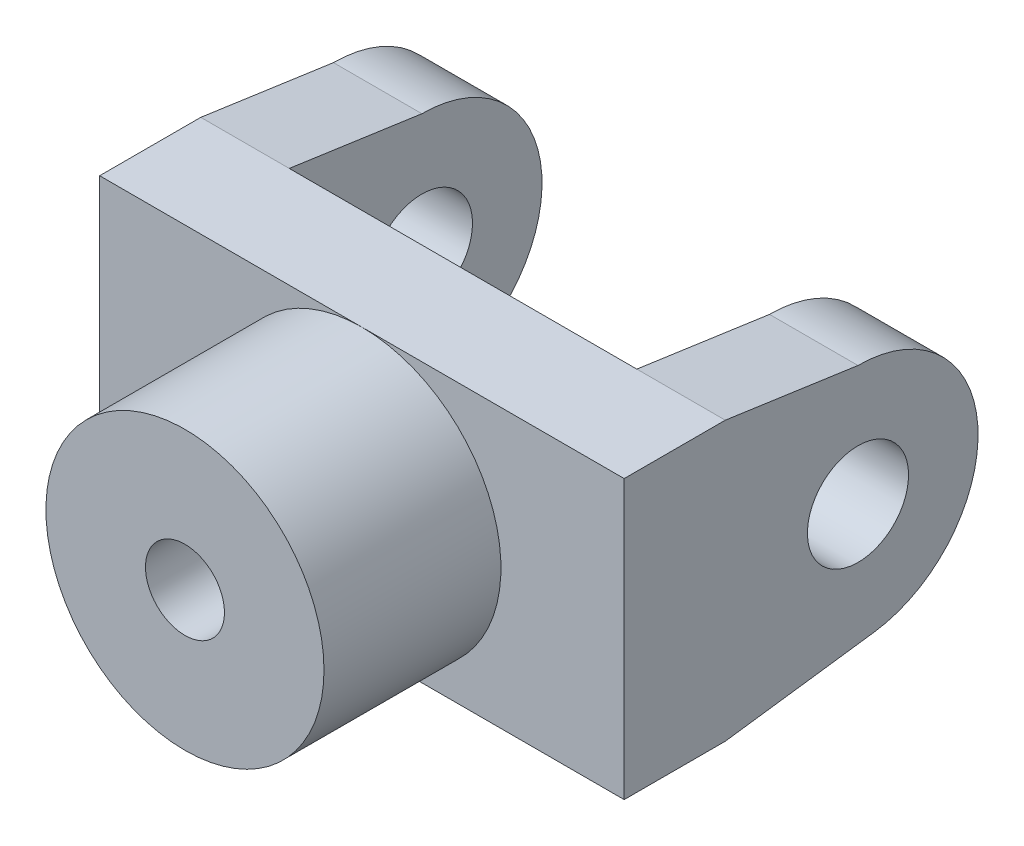
ISO-10303-21;
HEADER;
FILE_DESCRIPTION(('STEP AP214'),'2;1');
FILE_NAME('part.step','',(''),(''),'','','');
FILE_SCHEMA(('AUTOMOTIVE_DESIGN { 1 0 10303 214 1 1 1 1 }'));
ENDSEC;
DATA;
#1=APPLICATION_CONTEXT('core data for automotive mechanical design processes');
#2=APPLICATION_PROTOCOL_DEFINITION('international standard','automotive_design',2000,#1);
#3=PRODUCT_CONTEXT('',#1,'mechanical');
#4=PRODUCT('Part','Part','',(#3));
#5=PRODUCT_RELATED_PRODUCT_CATEGORY('part','',(#4));
#6=PRODUCT_DEFINITION_FORMATION('','',#4);
#7=PRODUCT_DEFINITION_CONTEXT('part definition',#1,'design');
#8=PRODUCT_DEFINITION('design','',#6,#7);
#9=PRODUCT_DEFINITION_SHAPE('','',#8);
#10=(LENGTH_UNIT() NAMED_UNIT(*) SI_UNIT(.MILLI.,.METRE.));
#11=(NAMED_UNIT(*) PLANE_ANGLE_UNIT() SI_UNIT($,.RADIAN.));
#12=(NAMED_UNIT(*) SI_UNIT($,.STERADIAN.) SOLID_ANGLE_UNIT());
#13=UNCERTAINTY_MEASURE_WITH_UNIT(LENGTH_MEASURE(1.E-05),#10,'distance_accuracy_value','');
#14=(GEOMETRIC_REPRESENTATION_CONTEXT(3) GLOBAL_UNCERTAINTY_ASSIGNED_CONTEXT((#13)) GLOBAL_UNIT_ASSIGNED_CONTEXT((#10,
#11,#12)) REPRESENTATION_CONTEXT('',''));
#15=CARTESIAN_POINT('',(0.,0.,0.));
#16=DIRECTION('',(0.,0.,1.));
#17=DIRECTION('',(1.,0.,0.));
#18=AXIS2_PLACEMENT_3D('',#15,#16,#17);
#19=CARTESIAN_POINT('',(0.,0.,0.));
#20=DIRECTION('',(0.,0.,1.));
#21=DIRECTION('',(1.,0.,0.));
#22=AXIS2_PLACEMENT_3D('',#19,#20,#21);
#23=PLANE('',#22);
#24=DIRECTION('',(0.,-1.,0.));
#25=VECTOR('',#24,1.);
#26=CARTESIAN_POINT('',(-55.,44.,0.));
#27=LINE('',#26,#25);
#28=CARTESIAN_POINT('',(-55.,44.,0.));
#29=VERTEX_POINT('',#28);
#30=CARTESIAN_POINT('',(-55.,-44.,0.));
#31=VERTEX_POINT('',#30);
#32=EDGE_CURVE('E141',#29,#31,#27,.T.);
#33=ORIENTED_EDGE('',*,*,#32,.F.);
#34=DIRECTION('',(-1.,0.,0.));
#35=VECTOR('',#34,1.);
#36=CARTESIAN_POINT('',(83.,44.,0.));
#37=LINE('',#36,#35);
#38=CARTESIAN_POINT('',(55.,44.,0.));
#39=VERTEX_POINT('',#38);
#40=EDGE_CURVE('E224',#39,#29,#37,.T.);
#41=ORIENTED_EDGE('',*,*,#40,.F.);
#42=DIRECTION('',(0.,-1.,0.));
#43=VECTOR('',#42,1.);
#44=CARTESIAN_POINT('',(55.,44.,0.));
#45=LINE('',#44,#43);
#46=CARTESIAN_POINT('',(55.,-44.,0.));
#47=VERTEX_POINT('',#46);
#48=EDGE_CURVE('E172',#39,#47,#45,.T.);
#49=ORIENTED_EDGE('',*,*,#48,.T.);
#50=DIRECTION('',(1.,0.,0.));
#51=VECTOR('',#50,1.);
#52=CARTESIAN_POINT('',(83.,-44.,0.));
#53=LINE('',#52,#51);
#54=EDGE_CURVE('E62',#31,#47,#53,.T.);
#55=ORIENTED_EDGE('',*,*,#54,.F.);
#56=EDGE_LOOP('',(#33,#41,#49,#55));
#57=FACE_BOUND('',#56,.T.);
#58=ADVANCED_FACE('F39',(#57),#23,.F.);
#59=CARTESIAN_POINT('',(0.,0.,32.));
#60=DIRECTION('',(0.,0.,1.));
#61=DIRECTION('',(1.,0.,0.));
#62=AXIS2_PLACEMENT_3D('',#59,#60,#61);
#63=PLANE('',#62);
#64=CARTESIAN_POINT('',(0.,0.,32.));
#65=DIRECTION('',(0.,0.,1.));
#66=DIRECTION('',(1.,0.,0.));
#67=AXIS2_PLACEMENT_3D('',#64,#65,#66);
#68=CIRCLE('',#67,44.);
#69=CARTESIAN_POINT('',(0.,44.,32.));
#70=VERTEX_POINT('',#69);
#71=CARTESIAN_POINT('',(0.,-44.,32.));
#72=VERTEX_POINT('',#71);
#73=EDGE_CURVE('E47',#70,#72,#68,.T.);
#74=ORIENTED_EDGE('',*,*,#73,.F.);
#75=DIRECTION('',(-1.,0.,0.));
#76=VECTOR('',#75,1.);
#77=CARTESIAN_POINT('',(83.,44.,32.));
#78=LINE('',#77,#76);
#79=CARTESIAN_POINT('',(-83.,44.,32.));
#80=VERTEX_POINT('',#79);
#81=EDGE_CURVE('E220',#70,#80,#78,.T.);
#82=ORIENTED_EDGE('',*,*,#81,.T.);
#83=DIRECTION('',(0.,-1.,0.));
#84=VECTOR('',#83,1.);
#85=CARTESIAN_POINT('',(-83.,-44.,32.));
#86=LINE('',#85,#84);
#87=CARTESIAN_POINT('',(-83.,-44.,32.));
#88=VERTEX_POINT('',#87);
#89=EDGE_CURVE('E210',#80,#88,#86,.T.);
#90=ORIENTED_EDGE('',*,*,#89,.T.);
#91=DIRECTION('',(1.,0.,0.));
#92=VECTOR('',#91,1.);
#93=CARTESIAN_POINT('',(83.,-44.,32.));
#94=LINE('',#93,#92);
#95=EDGE_CURVE('E215',#88,#72,#94,.T.);
#96=ORIENTED_EDGE('',*,*,#95,.T.);
#97=EDGE_LOOP('',(#74,#82,#90,#96));
#98=FACE_BOUND('',#97,.T.);
#99=ADVANCED_FACE('F254',(#98),#63,.T.);
#100=CARTESIAN_POINT('',(-83.,-44.,32.));
#101=DIRECTION('',(1.,0.,0.));
#102=DIRECTION('',(0.,0.,-1.));
#103=AXIS2_PLACEMENT_3D('',#100,#101,#102);
#104=PLANE('',#103);
#105=DIRECTION('',(0.,0.,-1.));
#106=VECTOR('',#105,1.);
#107=CARTESIAN_POINT('',(-83.,44.,32.));
#108=LINE('',#107,#106);
#109=CARTESIAN_POINT('',(-83.,44.,0.));
#110=VERTEX_POINT('',#109);
#111=EDGE_CURVE('E219',#80,#110,#108,.T.);
#112=ORIENTED_EDGE('',*,*,#111,.T.);
#113=DIRECTION('',(0.,0.141421356237309,0.989949493661166));
#114=VECTOR('',#113,1.);
#115=CARTESIAN_POINT('',(-83.,38.,-42.));
#116=LINE('',#115,#114);
#117=CARTESIAN_POINT('',(-83.,38.,-42.));
#118=VERTEX_POINT('',#117);
#119=EDGE_CURVE('E158',#118,#110,#116,.T.);
#120=ORIENTED_EDGE('',*,*,#119,.F.);
#121=CARTESIAN_POINT('',(-83.,0.,-42.));
#122=DIRECTION('',(1.,0.,0.));
#123=DIRECTION('',(0.,0.,-1.));
#124=AXIS2_PLACEMENT_3D('',#121,#122,#123);
#125=CIRCLE('',#124,38.);
#126=CARTESIAN_POINT('',(-83.,-37.6599459145,-47.072324291381));
#127=VERTEX_POINT('',#126);
#128=EDGE_CURVE('E137',#127,#118,#125,.T.);
#129=ORIENTED_EDGE('',*,*,#128,.F.);
#130=DIRECTION('',(0.,0.133482218194236,-0.991051208276316));
#131=VECTOR('',#130,1.);
#132=CARTESIAN_POINT('',(-83.,-44.,0.));
#133=LINE('',#132,#131);
#134=CARTESIAN_POINT('',(-83.,-44.,0.));
#135=VERTEX_POINT('',#134);
#136=EDGE_CURVE('E149',#135,#127,#133,.T.);
#137=ORIENTED_EDGE('',*,*,#136,.F.);
#138=DIRECTION('',(0.,0.,-1.));
#139=VECTOR('',#138,1.);
#140=CARTESIAN_POINT('',(-83.,-44.,32.));
#141=LINE('',#140,#139);
#142=EDGE_CURVE('E43',#88,#135,#141,.T.);
#143=ORIENTED_EDGE('',*,*,#142,.F.);
#144=ORIENTED_EDGE('',*,*,#89,.F.);
#145=EDGE_LOOP('',(#112,#120,#129,#137,#143,#144));
#146=FACE_BOUND('',#145,.T.);
#147=CARTESIAN_POINT('',(-83.,0.,-42.));
#148=DIRECTION('',(1.,0.,0.));
#149=DIRECTION('',(0.,0.,-1.));
#150=AXIS2_PLACEMENT_3D('',#147,#148,#149);
#151=CIRCLE('',#150,16.);
#152=CARTESIAN_POINT('',(-83.,0.,-58.));
#153=VERTEX_POINT('',#152);
#154=EDGE_CURVE('E153',#153,#153,#151,.T.);
#155=ORIENTED_EDGE('',*,*,#154,.T.);
#156=EDGE_LOOP('',(#155));
#157=FACE_BOUND('',#156,.T.);
#158=ADVANCED_FACE('F41',(#146,#157),#104,.F.);
#159=CARTESIAN_POINT('',(83.,-44.,32.));
#160=DIRECTION('',(0.,1.,0.));
#161=DIRECTION('',(-1.,0.,0.));
#162=AXIS2_PLACEMENT_3D('',#159,#160,#161);
#163=PLANE('',#162);
#164=EDGE_CURVE('E222',#135,#31,#53,.T.);
#165=ORIENTED_EDGE('',*,*,#164,.T.);
#166=ORIENTED_EDGE('',*,*,#54,.T.);
#167=DIRECTION('',(1.,0.,0.));
#168=VECTOR('',#167,1.);
#169=CARTESIAN_POINT('',(55.,-44.,0.));
#170=LINE('',#169,#168);
#171=CARTESIAN_POINT('',(83.,-44.,0.));
#172=VERTEX_POINT('',#171);
#173=EDGE_CURVE('E184',#47,#172,#170,.T.);
#174=ORIENTED_EDGE('',*,*,#173,.T.);
#175=DIRECTION('',(0.,0.,-1.));
#176=VECTOR('',#175,1.);
#177=CARTESIAN_POINT('',(83.,-44.,32.));
#178=LINE('',#177,#176);
#179=CARTESIAN_POINT('',(83.,-44.,32.));
#180=VERTEX_POINT('',#179);
#181=EDGE_CURVE('E229',#180,#172,#178,.T.);
#182=ORIENTED_EDGE('',*,*,#181,.F.);
#183=EDGE_CURVE('E209',#72,#180,#94,.T.);
#184=ORIENTED_EDGE('',*,*,#183,.F.);
#185=ORIENTED_EDGE('',*,*,#95,.F.);
#186=ORIENTED_EDGE('',*,*,#142,.T.);
#187=EDGE_LOOP('',(#165,#166,#174,#182,#184,#185,#186));
#188=FACE_BOUND('',#187,.T.);
#189=ADVANCED_FACE('F240',(#188),#163,.F.);
#190=CARTESIAN_POINT('',(83.,-44.,32.));
#191=DIRECTION('',(-1.,0.,0.));
#192=DIRECTION('',(0.,0.,1.));
#193=AXIS2_PLACEMENT_3D('',#190,#191,#192);
#194=PLANE('',#193);
#195=ORIENTED_EDGE('',*,*,#181,.T.);
#196=DIRECTION('',(0.,0.133482218194236,-0.991051208276316));
#197=VECTOR('',#196,1.);
#198=CARTESIAN_POINT('',(83.,-44.,0.));
#199=LINE('',#198,#197);
#200=CARTESIAN_POINT('',(83.,-37.6599459145,-47.072324291381));
#201=VERTEX_POINT('',#200);
#202=EDGE_CURVE('E190',#172,#201,#199,.T.);
#203=ORIENTED_EDGE('',*,*,#202,.T.);
#204=CARTESIAN_POINT('',(83.,0.,-42.));
#205=DIRECTION('',(1.,0.,0.));
#206=DIRECTION('',(0.,0.,-1.));
#207=AXIS2_PLACEMENT_3D('',#204,#205,#206);
#208=CIRCLE('',#207,38.);
#209=CARTESIAN_POINT('',(83.,38.,-42.));
#210=VERTEX_POINT('',#209);
#211=EDGE_CURVE('E174',#201,#210,#208,.T.);
#212=ORIENTED_EDGE('',*,*,#211,.T.);
#213=DIRECTION('',(0.,0.141421356237309,0.989949493661166));
#214=VECTOR('',#213,1.);
#215=CARTESIAN_POINT('',(83.,38.,-42.));
#216=LINE('',#215,#214);
#217=CARTESIAN_POINT('',(83.,44.,0.));
#218=VERTEX_POINT('',#217);
#219=EDGE_CURVE('E169',#210,#218,#216,.T.);
#220=ORIENTED_EDGE('',*,*,#219,.T.);
#221=DIRECTION('',(0.,0.,-1.));
#222=VECTOR('',#221,1.);
#223=CARTESIAN_POINT('',(83.,44.,32.));
#224=LINE('',#223,#222);
#225=CARTESIAN_POINT('',(83.,44.,32.));
#226=VERTEX_POINT('',#225);
#227=EDGE_CURVE('E226',#226,#218,#224,.T.);
#228=ORIENTED_EDGE('',*,*,#227,.F.);
#229=DIRECTION('',(0.,1.,0.));
#230=VECTOR('',#229,1.);
#231=CARTESIAN_POINT('',(83.,-44.,32.));
#232=LINE('',#231,#230);
#233=EDGE_CURVE('E214',#180,#226,#232,.T.);
#234=ORIENTED_EDGE('',*,*,#233,.F.);
#235=EDGE_LOOP('',(#195,#203,#212,#220,#228,#234));
#236=FACE_BOUND('',#235,.T.);
#237=CARTESIAN_POINT('',(83.,0.,-42.));
#238=DIRECTION('',(1.,0.,0.));
#239=DIRECTION('',(0.,0.,-1.));
#240=AXIS2_PLACEMENT_3D('',#237,#238,#239);
#241=CIRCLE('',#240,16.);
#242=CARTESIAN_POINT('',(83.,0.,-58.));
#243=VERTEX_POINT('',#242);
#244=EDGE_CURVE('E162',#243,#243,#241,.T.);
#245=ORIENTED_EDGE('',*,*,#244,.F.);
#246=EDGE_LOOP('',(#245));
#247=FACE_BOUND('',#246,.T.);
#248=ADVANCED_FACE('F275',(#236,#247),#194,.F.);
#249=CARTESIAN_POINT('',(83.,44.,32.));
#250=DIRECTION('',(0.,-1.,0.));
#251=DIRECTION('',(1.,0.,0.));
#252=AXIS2_PLACEMENT_3D('',#249,#250,#251);
#253=PLANE('',#252);
#254=EDGE_CURVE('E211',#218,#39,#37,.T.);
#255=ORIENTED_EDGE('',*,*,#254,.T.);
#256=ORIENTED_EDGE('',*,*,#40,.T.);
#257=DIRECTION('',(-1.,0.,0.));
#258=VECTOR('',#257,1.);
#259=CARTESIAN_POINT('',(-55.,44.,0.));
#260=LINE('',#259,#258);
#261=EDGE_CURVE('E150',#29,#110,#260,.T.);
#262=ORIENTED_EDGE('',*,*,#261,.T.);
#263=ORIENTED_EDGE('',*,*,#111,.F.);
#264=ORIENTED_EDGE('',*,*,#81,.F.);
#265=EDGE_CURVE('E217',#226,#70,#78,.T.);
#266=ORIENTED_EDGE('',*,*,#265,.F.);
#267=ORIENTED_EDGE('',*,*,#227,.T.);
#268=EDGE_LOOP('',(#255,#256,#262,#263,#264,#266,#267));
#269=FACE_BOUND('',#268,.T.);
#270=ADVANCED_FACE('F267',(#269),#253,.F.);
#271=EDGE_CURVE('E11',#72,#70,#68,.T.);
#272=ORIENTED_EDGE('',*,*,#271,.F.);
#273=ORIENTED_EDGE('',*,*,#183,.T.);
#274=ORIENTED_EDGE('',*,*,#233,.T.);
#275=ORIENTED_EDGE('',*,*,#265,.T.);
#276=EDGE_LOOP('',(#272,#273,#274,#275));
#277=FACE_BOUND('',#276,.T.);
#278=ADVANCED_FACE('F266',(#277),#63,.T.);
#279=CARTESIAN_POINT('',(0.,0.,88.));
#280=DIRECTION('',(0.,0.,1.));
#281=DIRECTION('',(1.,0.,0.));
#282=AXIS2_PLACEMENT_3D('',#279,#280,#281);
#283=PLANE('',#282);
#284=CARTESIAN_POINT('',(0.,0.,88.));
#285=DIRECTION('',(0.,0.,1.));
#286=DIRECTION('',(1.,0.,0.));
#287=AXIS2_PLACEMENT_3D('',#284,#285,#286);
#288=CIRCLE('',#287,44.);
#289=CARTESIAN_POINT('',(44.,0.,88.));
#290=VERTEX_POINT('',#289);
#291=EDGE_CURVE('E201',#290,#290,#288,.T.);
#292=ORIENTED_EDGE('',*,*,#291,.T.);
#293=EDGE_LOOP('',(#292));
#294=FACE_BOUND('',#293,.T.);
#295=CARTESIAN_POINT('',(0.,0.,88.));
#296=DIRECTION('',(0.,0.,1.));
#297=DIRECTION('',(1.,0.,0.));
#298=AXIS2_PLACEMENT_3D('',#295,#296,#297);
#299=CIRCLE('',#298,12.5);
#300=CARTESIAN_POINT('',(12.5,0.,88.));
#301=VERTEX_POINT('',#300);
#302=EDGE_CURVE('E196',#301,#301,#299,.T.);
#303=ORIENTED_EDGE('',*,*,#302,.F.);
#304=EDGE_LOOP('',(#303));
#305=FACE_BOUND('',#304,.T.);
#306=ADVANCED_FACE('F344',(#294,#305),#283,.T.);
#307=CARTESIAN_POINT('',(0.,0.,88.));
#308=DIRECTION('',(0.,0.,-1.));
#309=DIRECTION('',(-1.,0.,0.));
#310=AXIS2_PLACEMENT_3D('',#307,#308,#309);
#311=CYLINDRICAL_SURFACE('',#310,44.);
#312=ORIENTED_EDGE('',*,*,#291,.F.);
#313=EDGE_LOOP('',(#312));
#314=FACE_BOUND('',#313,.T.);
#315=ORIENTED_EDGE('',*,*,#73,.T.);
#316=ORIENTED_EDGE('',*,*,#271,.T.);
#317=EDGE_LOOP('',(#315,#316));
#318=FACE_BOUND('',#317,.T.);
#319=ADVANCED_FACE('F366',(#314,#318),#311,.T.);
#320=CARTESIAN_POINT('',(0.,0.,88.));
#321=DIRECTION('',(0.,0.,-1.));
#322=DIRECTION('',(-1.,0.,0.));
#323=AXIS2_PLACEMENT_3D('',#320,#321,#322);
#324=CYLINDRICAL_SURFACE('',#323,12.5);
#325=ORIENTED_EDGE('',*,*,#302,.T.);
#326=EDGE_LOOP('',(#325));
#327=FACE_BOUND('',#326,.T.);
#328=CARTESIAN_POINT('',(0.,0.,32.));
#329=DIRECTION('',(0.,0.,1.));
#330=DIRECTION('',(1.,0.,0.));
#331=AXIS2_PLACEMENT_3D('',#328,#329,#330);
#332=CIRCLE('',#331,12.5);
#333=CARTESIAN_POINT('',(12.5,0.,32.));
#334=VERTEX_POINT('',#333);
#335=EDGE_CURVE('E192',#334,#334,#332,.T.);
#336=ORIENTED_EDGE('',*,*,#335,.F.);
#337=EDGE_LOOP('',(#336));
#338=FACE_BOUND('',#337,.T.);
#339=ADVANCED_FACE('F358',(#327,#338),#324,.F.);
#340=ORIENTED_EDGE('',*,*,#335,.T.);
#341=EDGE_LOOP('',(#340));
#342=FACE_BOUND('',#341,.T.);
#343=ADVANCED_FACE('F264',(#342),#63,.T.);
#344=CARTESIAN_POINT('',(55.,38.,-42.));
#345=DIRECTION('',(0.,0.989949493661167,-0.141421356237309));
#346=DIRECTION('',(0.,0.141421356237309,0.989949493661167));
#347=AXIS2_PLACEMENT_3D('',#344,#345,#346);
#348=PLANE('',#347);
#349=ORIENTED_EDGE('',*,*,#219,.F.);
#350=DIRECTION('',(1.,0.,0.));
#351=VECTOR('',#350,1.);
#352=CARTESIAN_POINT('',(55.,38.,-42.));
#353=LINE('',#352,#351);
#354=CARTESIAN_POINT('',(55.,38.,-42.));
#355=VERTEX_POINT('',#354);
#356=EDGE_CURVE('E195',#355,#210,#353,.T.);
#357=ORIENTED_EDGE('',*,*,#356,.F.);
#358=DIRECTION('',(0.,0.141421356237309,0.989949493661166));
#359=VECTOR('',#358,1.);
#360=CARTESIAN_POINT('',(55.,38.,-42.));
#361=LINE('',#360,#359);
#362=EDGE_CURVE('E173',#355,#39,#361,.T.);
#363=ORIENTED_EDGE('',*,*,#362,.T.);
#364=ORIENTED_EDGE('',*,*,#254,.F.);
#365=EDGE_LOOP('',(#349,#357,#363,#364));
#366=FACE_BOUND('',#365,.T.);
#367=ADVANCED_FACE('F354',(#366),#348,.T.);
#368=CARTESIAN_POINT('',(55.,0.,-42.));
#369=DIRECTION('',(1.,0.,0.));
#370=DIRECTION('',(0.,0.,-1.));
#371=AXIS2_PLACEMENT_3D('',#368,#369,#370);
#372=CYLINDRICAL_SURFACE('',#371,38.);
#373=ORIENTED_EDGE('',*,*,#211,.F.);
#374=DIRECTION('',(1.,0.,0.));
#375=VECTOR('',#374,1.);
#376=CARTESIAN_POINT('',(55.,-37.6599459145,-47.072324291381));
#377=LINE('',#376,#375);
#378=CARTESIAN_POINT('',(55.,-37.6599459145,-47.072324291381));
#379=VERTEX_POINT('',#378);
#380=EDGE_CURVE('E194',#379,#201,#377,.T.);
#381=ORIENTED_EDGE('',*,*,#380,.F.);
#382=CARTESIAN_POINT('',(55.,0.,-42.));
#383=DIRECTION('',(1.,0.,0.));
#384=DIRECTION('',(0.,0.,-1.));
#385=AXIS2_PLACEMENT_3D('',#382,#383,#384);
#386=CIRCLE('',#385,38.);
#387=EDGE_CURVE('E182',#379,#355,#386,.T.);
#388=ORIENTED_EDGE('',*,*,#387,.T.);
#389=ORIENTED_EDGE('',*,*,#356,.T.);
#390=EDGE_LOOP('',(#373,#381,#388,#389));
#391=FACE_BOUND('',#390,.T.);
#392=ADVANCED_FACE('F396',(#391),#372,.T.);
#393=CARTESIAN_POINT('',(55.,-44.,0.));
#394=DIRECTION('',(0.,-0.991051208276316,-0.133482218194236));
#395=DIRECTION('',(0.,0.133482218194236,-0.991051208276316));
#396=AXIS2_PLACEMENT_3D('',#393,#394,#395);
#397=PLANE('',#396);
#398=ORIENTED_EDGE('',*,*,#202,.F.);
#399=ORIENTED_EDGE('',*,*,#173,.F.);
#400=DIRECTION('',(0.,0.133482218194236,-0.991051208276316));
#401=VECTOR('',#400,1.);
#402=CARTESIAN_POINT('',(55.,-44.,0.));
#403=LINE('',#402,#401);
#404=EDGE_CURVE('E176',#47,#379,#403,.T.);
#405=ORIENTED_EDGE('',*,*,#404,.T.);
#406=ORIENTED_EDGE('',*,*,#380,.T.);
#407=EDGE_LOOP('',(#398,#399,#405,#406));
#408=FACE_BOUND('',#407,.T.);
#409=ADVANCED_FACE('F406',(#408),#397,.T.);
#410=CARTESIAN_POINT('',(55.,0.,-42.));
#411=DIRECTION('',(1.,0.,0.));
#412=DIRECTION('',(0.,0.,-1.));
#413=AXIS2_PLACEMENT_3D('',#410,#411,#412);
#414=PLANE('',#413);
#415=CARTESIAN_POINT('',(55.,0.,-42.));
#416=DIRECTION('',(1.,0.,0.));
#417=DIRECTION('',(0.,0.,-1.));
#418=AXIS2_PLACEMENT_3D('',#415,#416,#417);
#419=CIRCLE('',#418,16.);
#420=CARTESIAN_POINT('',(55.,0.,-58.));
#421=VERTEX_POINT('',#420);
#422=EDGE_CURVE('E164',#421,#421,#419,.T.);
#423=ORIENTED_EDGE('',*,*,#422,.T.);
#424=EDGE_LOOP('',(#423));
#425=FACE_BOUND('',#424,.T.);
#426=ORIENTED_EDGE('',*,*,#362,.F.);
#427=ORIENTED_EDGE('',*,*,#387,.F.);
#428=ORIENTED_EDGE('',*,*,#404,.F.);
#429=ORIENTED_EDGE('',*,*,#48,.F.);
#430=EDGE_LOOP('',(#426,#427,#428,#429));
#431=FACE_BOUND('',#430,.T.);
#432=ADVANCED_FACE('F416',(#425,#431),#414,.F.);
#433=CARTESIAN_POINT('',(55.,0.,-42.));
#434=DIRECTION('',(1.,0.,0.));
#435=DIRECTION('',(0.,0.,-1.));
#436=AXIS2_PLACEMENT_3D('',#433,#434,#435);
#437=CYLINDRICAL_SURFACE('',#436,16.);
#438=ORIENTED_EDGE('',*,*,#422,.F.);
#439=EDGE_LOOP('',(#438));
#440=FACE_BOUND('',#439,.T.);
#441=ORIENTED_EDGE('',*,*,#244,.T.);
#442=EDGE_LOOP('',(#441));
#443=FACE_BOUND('',#442,.T.);
#444=ADVANCED_FACE('F298',(#440,#443),#437,.F.);
#445=CARTESIAN_POINT('',(-55.,0.,-42.));
#446=DIRECTION('',(-1.,0.,0.));
#447=DIRECTION('',(0.,0.,-1.));
#448=AXIS2_PLACEMENT_3D('',#445,#446,#447);
#449=PLANE('',#448);
#450=DIRECTION('',(0.,0.141421356237309,0.989949493661166));
#451=VECTOR('',#450,1.);
#452=CARTESIAN_POINT('',(-55.,38.,-42.));
#453=LINE('',#452,#451);
#454=CARTESIAN_POINT('',(-55.,38.,-42.));
#455=VERTEX_POINT('',#454);
#456=EDGE_CURVE('E128',#455,#29,#453,.T.);
#457=ORIENTED_EDGE('',*,*,#456,.T.);
#458=ORIENTED_EDGE('',*,*,#32,.T.);
#459=DIRECTION('',(0.,0.133482218194236,-0.991051208276316));
#460=VECTOR('',#459,1.);
#461=CARTESIAN_POINT('',(-55.,-44.,0.));
#462=LINE('',#461,#460);
#463=CARTESIAN_POINT('',(-55.,-37.6599459145,-47.072324291381));
#464=VERTEX_POINT('',#463);
#465=EDGE_CURVE('E57',#31,#464,#462,.T.);
#466=ORIENTED_EDGE('',*,*,#465,.T.);
#467=CARTESIAN_POINT('',(-55.,0.,-42.));
#468=DIRECTION('',(1.,0.,0.));
#469=DIRECTION('',(0.,0.,-1.));
#470=AXIS2_PLACEMENT_3D('',#467,#468,#469);
#471=CIRCLE('',#470,38.);
#472=EDGE_CURVE('E124',#464,#455,#471,.T.);
#473=ORIENTED_EDGE('',*,*,#472,.T.);
#474=EDGE_LOOP('',(#457,#458,#466,#473));
#475=FACE_BOUND('',#474,.T.);
#476=CARTESIAN_POINT('',(-55.,0.,-42.));
#477=DIRECTION('',(1.,0.,0.));
#478=DIRECTION('',(0.,0.,-1.));
#479=AXIS2_PLACEMENT_3D('',#476,#477,#478);
#480=CIRCLE('',#479,16.);
#481=CARTESIAN_POINT('',(-55.,0.,-58.));
#482=VERTEX_POINT('',#481);
#483=EDGE_CURVE('E159',#482,#482,#480,.T.);
#484=ORIENTED_EDGE('',*,*,#483,.F.);
#485=EDGE_LOOP('',(#484));
#486=FACE_BOUND('',#485,.T.);
#487=ADVANCED_FACE('F130',(#475,#486),#449,.F.);
#488=CARTESIAN_POINT('',(-55.,38.,-42.));
#489=DIRECTION('',(0.,-0.989949493661167,0.141421356237309));
#490=DIRECTION('',(0.,-0.141421356237309,-0.989949493661167));
#491=AXIS2_PLACEMENT_3D('',#488,#489,#490);
#492=PLANE('',#491);
#493=ORIENTED_EDGE('',*,*,#119,.T.);
#494=ORIENTED_EDGE('',*,*,#261,.F.);
#495=ORIENTED_EDGE('',*,*,#456,.F.);
#496=DIRECTION('',(-1.,0.,0.));
#497=VECTOR('',#496,1.);
#498=CARTESIAN_POINT('',(-55.,38.,-42.));
#499=LINE('',#498,#497);
#500=EDGE_CURVE('E138',#455,#118,#499,.T.);
#501=ORIENTED_EDGE('',*,*,#500,.T.);
#502=EDGE_LOOP('',(#493,#494,#495,#501));
#503=FACE_BOUND('',#502,.T.);
#504=ADVANCED_FACE('F144',(#503),#492,.F.);
#505=CARTESIAN_POINT('',(-55.,-44.,0.));
#506=DIRECTION('',(0.,0.991051208276316,0.133482218194236));
#507=DIRECTION('',(0.,-0.133482218194236,0.991051208276316));
#508=AXIS2_PLACEMENT_3D('',#505,#506,#507);
#509=PLANE('',#508);
#510=ORIENTED_EDGE('',*,*,#136,.T.);
#511=DIRECTION('',(-1.,0.,0.));
#512=VECTOR('',#511,1.);
#513=CARTESIAN_POINT('',(-55.,-37.6599459145,-47.072324291381));
#514=LINE('',#513,#512);
#515=EDGE_CURVE('E142',#464,#127,#514,.T.);
#516=ORIENTED_EDGE('',*,*,#515,.F.);
#517=ORIENTED_EDGE('',*,*,#465,.F.);
#518=ORIENTED_EDGE('',*,*,#164,.F.);
#519=EDGE_LOOP('',(#510,#516,#517,#518));
#520=FACE_BOUND('',#519,.T.);
#521=ADVANCED_FACE('F241',(#520),#509,.F.);
#522=CARTESIAN_POINT('',(-55.,0.,-42.));
#523=DIRECTION('',(-1.,0.,0.));
#524=DIRECTION('',(0.,0.,1.));
#525=AXIS2_PLACEMENT_3D('',#522,#523,#524);
#526=CYLINDRICAL_SURFACE('',#525,38.);
#527=ORIENTED_EDGE('',*,*,#128,.T.);
#528=ORIENTED_EDGE('',*,*,#500,.F.);
#529=ORIENTED_EDGE('',*,*,#472,.F.);
#530=ORIENTED_EDGE('',*,*,#515,.T.);
#531=EDGE_LOOP('',(#527,#528,#529,#530));
#532=FACE_BOUND('',#531,.T.);
#533=ADVANCED_FACE('F140',(#532),#526,.T.);
#534=CARTESIAN_POINT('',(-55.,0.,-42.));
#535=DIRECTION('',(-1.,0.,0.));
#536=DIRECTION('',(0.,0.,1.));
#537=AXIS2_PLACEMENT_3D('',#534,#535,#536);
#538=CYLINDRICAL_SURFACE('',#537,16.);
#539=ORIENTED_EDGE('',*,*,#483,.T.);
#540=EDGE_LOOP('',(#539));
#541=FACE_BOUND('',#540,.T.);
#542=ORIENTED_EDGE('',*,*,#154,.F.);
#543=EDGE_LOOP('',(#542));
#544=FACE_BOUND('',#543,.T.);
#545=ADVANCED_FACE('F249',(#541,#544),#538,.F.);
#546=CLOSED_SHELL('',(#58,#99,#158,#189,#248,#270,#278,#306,#319,#339,#343,#367,#392,#409,#432,
#444,#487,#504,#521,#533,#545));
#547=MANIFOLD_SOLID_BREP('B2',#546);
#548=ADVANCED_BREP_SHAPE_REPRESENTATION('',(#18,#547),#14);
#549=SHAPE_DEFINITION_REPRESENTATION(#9,#548);
ENDSEC;
END-ISO-10303-21;
